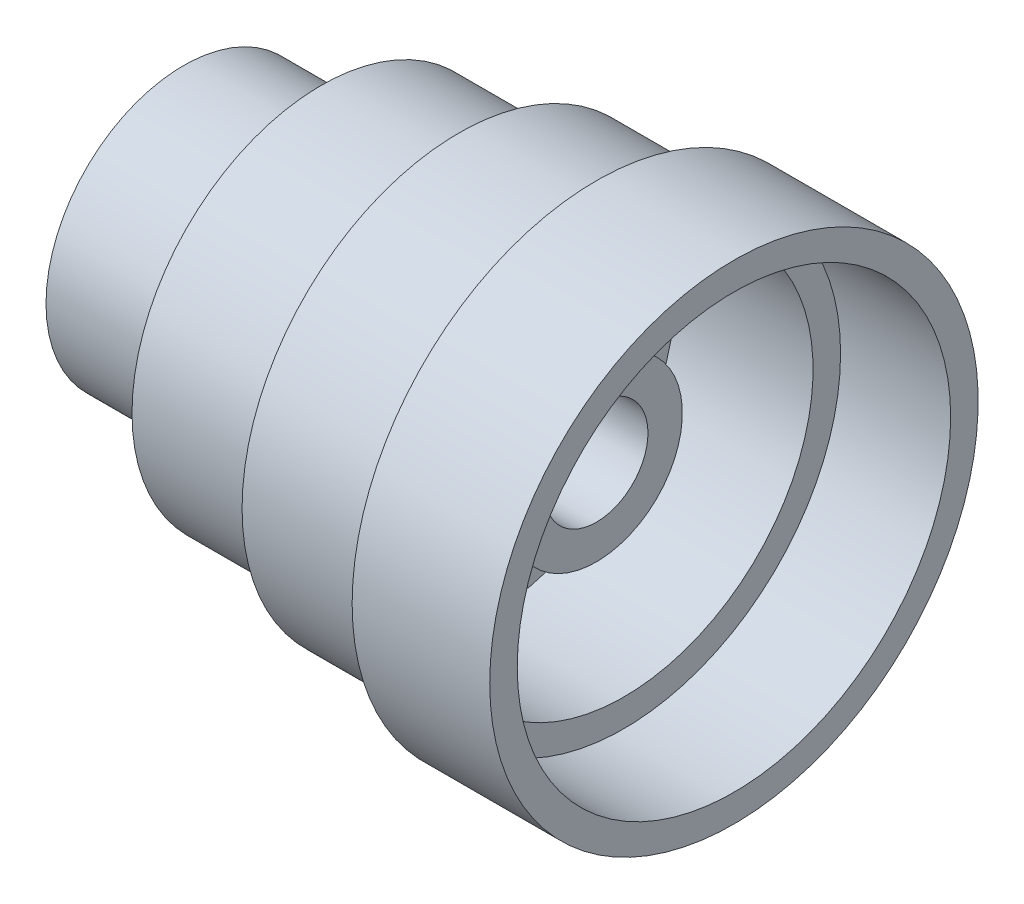
ISO-10303-21;
HEADER;
FILE_DESCRIPTION(('STEP AP214'),'2;1');
FILE_NAME('part.step','',(''),(''),'','','');
FILE_SCHEMA(('AUTOMOTIVE_DESIGN { 1 0 10303 214 1 1 1 1 }'));
ENDSEC;
DATA;
#1=APPLICATION_CONTEXT('core data for automotive mechanical design processes');
#2=APPLICATION_PROTOCOL_DEFINITION('international standard','automotive_design',2000,#1);
#3=PRODUCT_CONTEXT('',#1,'mechanical');
#4=PRODUCT('Part','Part','',(#3));
#5=PRODUCT_RELATED_PRODUCT_CATEGORY('part','',(#4));
#6=PRODUCT_DEFINITION_FORMATION('','',#4);
#7=PRODUCT_DEFINITION_CONTEXT('part definition',#1,'design');
#8=PRODUCT_DEFINITION('design','',#6,#7);
#9=PRODUCT_DEFINITION_SHAPE('','',#8);
#10=(LENGTH_UNIT() NAMED_UNIT(*) SI_UNIT(.MILLI.,.METRE.));
#11=(NAMED_UNIT(*) PLANE_ANGLE_UNIT() SI_UNIT($,.RADIAN.));
#12=(NAMED_UNIT(*) SI_UNIT($,.STERADIAN.) SOLID_ANGLE_UNIT());
#13=UNCERTAINTY_MEASURE_WITH_UNIT(LENGTH_MEASURE(1.E-05),#10,'distance_accuracy_value','');
#14=(GEOMETRIC_REPRESENTATION_CONTEXT(3) GLOBAL_UNCERTAINTY_ASSIGNED_CONTEXT((#13)) GLOBAL_UNIT_ASSIGNED_CONTEXT((#10,
#11,#12)) REPRESENTATION_CONTEXT('',''));
#15=CARTESIAN_POINT('',(0.,0.,0.));
#16=DIRECTION('',(0.,0.,1.));
#17=DIRECTION('',(1.,0.,0.));
#18=AXIS2_PLACEMENT_3D('',#15,#16,#17);
#19=CARTESIAN_POINT('',(-51.5789473684211,0.,0.));
#20=DIRECTION('',(-1.,0.,0.));
#21=DIRECTION('',(0.,0.,1.));
#22=AXIS2_PLACEMENT_3D('',#19,#20,#21);
#23=CYLINDRICAL_SURFACE('',#22,15.);
#24=CARTESIAN_POINT('',(0.,0.,0.));
#25=DIRECTION('',(-1.,0.,0.));
#26=DIRECTION('',(0.,0.,1.));
#27=AXIS2_PLACEMENT_3D('',#24,#25,#26);
#28=CIRCLE('',#27,15.);
#29=CARTESIAN_POINT('',(0.,14.6969384566991,-3.));
#30=VERTEX_POINT('',#29);
#31=CARTESIAN_POINT('',(0.,14.6969384566991,3.));
#32=VERTEX_POINT('',#31);
#33=EDGE_CURVE('E98',#30,#32,#28,.T.);
#34=ORIENTED_EDGE('',*,*,#33,.T.);
#35=DIRECTION('',(-1.,0.,0.));
#36=VECTOR('',#35,1.);
#37=CARTESIAN_POINT('',(-51.5789473684211,14.6969384566991,3.));
#38=LINE('',#37,#36);
#39=CARTESIAN_POINT('',(120.,14.6969384566991,3.));
#40=VERTEX_POINT('',#39);
#41=EDGE_CURVE('E110',#32,#40,#38,.F.);
#42=ORIENTED_EDGE('',*,*,#41,.T.);
#43=CARTESIAN_POINT('',(120.,0.,0.));
#44=DIRECTION('',(-1.,0.,0.));
#45=DIRECTION('',(0.,0.,1.));
#46=AXIS2_PLACEMENT_3D('',#43,#44,#45);
#47=CIRCLE('',#46,15.);
#48=CARTESIAN_POINT('',(120.,14.6969384566991,-3.));
#49=VERTEX_POINT('',#48);
#50=EDGE_CURVE('E46',#49,#40,#47,.T.);
#51=ORIENTED_EDGE('',*,*,#50,.F.);
#52=DIRECTION('',(-1.,0.,0.));
#53=VECTOR('',#52,1.);
#54=CARTESIAN_POINT('',(-51.5789473684211,14.6969384566991,-3.));
#55=LINE('',#54,#53);
#56=EDGE_CURVE('E102',#49,#30,#55,.T.);
#57=ORIENTED_EDGE('',*,*,#56,.T.);
#58=EDGE_LOOP('',(#34,#42,#51,#57));
#59=FACE_BOUND('',#58,.T.);
#60=ADVANCED_FACE('F39',(#59),#23,.F.);
#61=CARTESIAN_POINT('',(120.,25.,0.));
#62=DIRECTION('',(-1.,0.,0.));
#63=DIRECTION('',(0.,0.,1.));
#64=AXIS2_PLACEMENT_3D('',#61,#62,#63);
#65=PLANE('',#64);
#66=ORIENTED_EDGE('',*,*,#50,.T.);
#67=DIRECTION('',(0.,1.,0.));
#68=VECTOR('',#67,1.);
#69=CARTESIAN_POINT('',(120.,25.,3.));
#70=LINE('',#69,#68);
#71=CARTESIAN_POINT('',(120.,18.,3.));
#72=VERTEX_POINT('',#71);
#73=EDGE_CURVE('E58',#40,#72,#70,.T.);
#74=ORIENTED_EDGE('',*,*,#73,.T.);
#75=DIRECTION('',(0.,0.,-1.));
#76=VECTOR('',#75,1.);
#77=CARTESIAN_POINT('',(120.,18.,0.));
#78=LINE('',#77,#76);
#79=CARTESIAN_POINT('',(120.,18.,-3.));
#80=VERTEX_POINT('',#79);
#81=EDGE_CURVE('E87',#72,#80,#78,.T.);
#82=ORIENTED_EDGE('',*,*,#81,.T.);
#83=DIRECTION('',(0.,-1.,0.));
#84=VECTOR('',#83,1.);
#85=CARTESIAN_POINT('',(120.,25.,-3.));
#86=LINE('',#85,#84);
#87=EDGE_CURVE('E83',#80,#49,#86,.T.);
#88=ORIENTED_EDGE('',*,*,#87,.T.);
#89=EDGE_LOOP('',(#66,#74,#82,#88));
#90=FACE_BOUND('',#89,.T.);
#91=CARTESIAN_POINT('',(120.,0.,0.));
#92=DIRECTION('',(-1.,0.,0.));
#93=DIRECTION('',(0.,0.,1.));
#94=AXIS2_PLACEMENT_3D('',#91,#92,#93);
#95=CIRCLE('',#94,25.);
#96=CARTESIAN_POINT('',(120.,0.,25.));
#97=VERTEX_POINT('',#96);
#98=EDGE_CURVE('E154',#97,#97,#95,.T.);
#99=ORIENTED_EDGE('',*,*,#98,.F.);
#100=EDGE_LOOP('',(#99));
#101=FACE_BOUND('',#100,.T.);
#102=ADVANCED_FACE('F159',(#90,#101),#65,.F.);
#103=CARTESIAN_POINT('',(-51.5789473684211,0.,0.));
#104=DIRECTION('',(-1.,0.,0.));
#105=DIRECTION('',(0.,0.,1.));
#106=AXIS2_PLACEMENT_3D('',#103,#104,#105);
#107=CYLINDRICAL_SURFACE('',#106,25.);
#108=CARTESIAN_POINT('',(48.,0.,0.));
#109=DIRECTION('',(-1.,0.,0.));
#110=DIRECTION('',(0.,0.,1.));
#111=AXIS2_PLACEMENT_3D('',#108,#109,#110);
#112=CIRCLE('',#111,25.);
#113=CARTESIAN_POINT('',(48.,0.,25.));
#114=VERTEX_POINT('',#113);
#115=EDGE_CURVE('E155',#114,#114,#112,.T.);
#116=ORIENTED_EDGE('',*,*,#115,.F.);
#117=EDGE_LOOP('',(#116));
#118=FACE_BOUND('',#117,.T.);
#119=ORIENTED_EDGE('',*,*,#98,.T.);
#120=EDGE_LOOP('',(#119));
#121=FACE_BOUND('',#120,.T.);
#122=ADVANCED_FACE('F176',(#118,#121),#107,.T.);
#123=CARTESIAN_POINT('',(48.,40.,0.));
#124=DIRECTION('',(-1.,0.,0.));
#125=DIRECTION('',(0.,0.,1.));
#126=AXIS2_PLACEMENT_3D('',#123,#124,#125);
#127=PLANE('',#126);
#128=CARTESIAN_POINT('',(48.,0.,0.));
#129=DIRECTION('',(-1.,0.,0.));
#130=DIRECTION('',(0.,0.,1.));
#131=AXIS2_PLACEMENT_3D('',#128,#129,#130);
#132=CIRCLE('',#131,40.);
#133=CARTESIAN_POINT('',(48.,0.,40.));
#134=VERTEX_POINT('',#133);
#135=EDGE_CURVE('E149',#134,#134,#132,.T.);
#136=ORIENTED_EDGE('',*,*,#135,.F.);
#137=EDGE_LOOP('',(#136));
#138=FACE_BOUND('',#137,.T.);
#139=ORIENTED_EDGE('',*,*,#115,.T.);
#140=EDGE_LOOP('',(#139));
#141=FACE_BOUND('',#140,.T.);
#142=ADVANCED_FACE('F181',(#138,#141),#127,.F.);
#143=CARTESIAN_POINT('',(-51.5789473684211,0.,0.));
#144=DIRECTION('',(-1.,0.,0.));
#145=DIRECTION('',(0.,0.,1.));
#146=AXIS2_PLACEMENT_3D('',#143,#144,#145);
#147=CYLINDRICAL_SURFACE('',#146,40.);
#148=CARTESIAN_POINT('',(88.,0.,0.));
#149=DIRECTION('',(-1.,0.,0.));
#150=DIRECTION('',(0.,0.,1.));
#151=AXIS2_PLACEMENT_3D('',#148,#149,#150);
#152=CIRCLE('',#151,40.);
#153=CARTESIAN_POINT('',(88.,0.,40.));
#154=VERTEX_POINT('',#153);
#155=EDGE_CURVE('E148',#154,#154,#152,.T.);
#156=ORIENTED_EDGE('',*,*,#155,.F.);
#157=EDGE_LOOP('',(#156));
#158=FACE_BOUND('',#157,.T.);
#159=ORIENTED_EDGE('',*,*,#135,.T.);
#160=EDGE_LOOP('',(#159));
#161=FACE_BOUND('',#160,.T.);
#162=ADVANCED_FACE('F186',(#158,#161),#147,.F.);
#163=CARTESIAN_POINT('',(88.,55.,0.));
#164=DIRECTION('',(-1.,0.,0.));
#165=DIRECTION('',(0.,0.,1.));
#166=AXIS2_PLACEMENT_3D('',#163,#164,#165);
#167=PLANE('',#166);
#168=CARTESIAN_POINT('',(88.,0.,0.));
#169=DIRECTION('',(-1.,0.,0.));
#170=DIRECTION('',(0.,0.,1.));
#171=AXIS2_PLACEMENT_3D('',#168,#169,#170);
#172=CIRCLE('',#171,55.);
#173=CARTESIAN_POINT('',(88.,0.,55.));
#174=VERTEX_POINT('',#173);
#175=EDGE_CURVE('E141',#174,#174,#172,.T.);
#176=ORIENTED_EDGE('',*,*,#175,.F.);
#177=EDGE_LOOP('',(#176));
#178=FACE_BOUND('',#177,.T.);
#179=ORIENTED_EDGE('',*,*,#155,.T.);
#180=EDGE_LOOP('',(#179));
#181=FACE_BOUND('',#180,.T.);
#182=ADVANCED_FACE('F195',(#178,#181),#167,.F.);
#183=CARTESIAN_POINT('',(-51.5789473684211,0.,0.));
#184=DIRECTION('',(-1.,0.,0.));
#185=DIRECTION('',(0.,0.,1.));
#186=AXIS2_PLACEMENT_3D('',#183,#184,#185);
#187=CYLINDRICAL_SURFACE('',#186,55.);
#188=CARTESIAN_POINT('',(128.,0.,0.));
#189=DIRECTION('',(-1.,0.,0.));
#190=DIRECTION('',(0.,0.,1.));
#191=AXIS2_PLACEMENT_3D('',#188,#189,#190);
#192=CIRCLE('',#191,55.);
#193=CARTESIAN_POINT('',(128.,0.,55.));
#194=VERTEX_POINT('',#193);
#195=EDGE_CURVE('E138',#194,#194,#192,.T.);
#196=ORIENTED_EDGE('',*,*,#195,.F.);
#197=EDGE_LOOP('',(#196));
#198=FACE_BOUND('',#197,.T.);
#199=ORIENTED_EDGE('',*,*,#175,.T.);
#200=EDGE_LOOP('',(#199));
#201=FACE_BOUND('',#200,.T.);
#202=ADVANCED_FACE('F197',(#198,#201),#187,.F.);
#203=CARTESIAN_POINT('',(128.,63.,0.));
#204=DIRECTION('',(-1.,0.,0.));
#205=DIRECTION('',(0.,0.,1.));
#206=AXIS2_PLACEMENT_3D('',#203,#204,#205);
#207=PLANE('',#206);
#208=CARTESIAN_POINT('',(128.,0.,0.));
#209=DIRECTION('',(-1.,0.,0.));
#210=DIRECTION('',(0.,0.,1.));
#211=AXIS2_PLACEMENT_3D('',#208,#209,#210);
#212=CIRCLE('',#211,63.);
#213=CARTESIAN_POINT('',(128.,0.,63.));
#214=VERTEX_POINT('',#213);
#215=EDGE_CURVE('E139',#214,#214,#212,.T.);
#216=ORIENTED_EDGE('',*,*,#215,.F.);
#217=EDGE_LOOP('',(#216));
#218=FACE_BOUND('',#217,.T.);
#219=ORIENTED_EDGE('',*,*,#195,.T.);
#220=EDGE_LOOP('',(#219));
#221=FACE_BOUND('',#220,.T.);
#222=ADVANCED_FACE('F203',(#218,#221),#207,.F.);
#223=CARTESIAN_POINT('',(-51.5789473684211,0.,0.));
#224=DIRECTION('',(-1.,0.,0.));
#225=DIRECTION('',(0.,0.,1.));
#226=AXIS2_PLACEMENT_3D('',#223,#224,#225);
#227=CYLINDRICAL_SURFACE('',#226,63.);
#228=CARTESIAN_POINT('',(160.,0.,0.));
#229=DIRECTION('',(-1.,0.,0.));
#230=DIRECTION('',(0.,0.,1.));
#231=AXIS2_PLACEMENT_3D('',#228,#229,#230);
#232=CIRCLE('',#231,63.);
#233=CARTESIAN_POINT('',(160.,0.,63.));
#234=VERTEX_POINT('',#233);
#235=EDGE_CURVE('E131',#234,#234,#232,.T.);
#236=ORIENTED_EDGE('',*,*,#235,.F.);
#237=EDGE_LOOP('',(#236));
#238=FACE_BOUND('',#237,.T.);
#239=ORIENTED_EDGE('',*,*,#215,.T.);
#240=EDGE_LOOP('',(#239));
#241=FACE_BOUND('',#240,.T.);
#242=ADVANCED_FACE('F202',(#238,#241),#227,.F.);
#243=CARTESIAN_POINT('',(160.,71.,0.));
#244=DIRECTION('',(-1.,0.,0.));
#245=DIRECTION('',(0.,0.,1.));
#246=AXIS2_PLACEMENT_3D('',#243,#244,#245);
#247=PLANE('',#246);
#248=CARTESIAN_POINT('',(160.,0.,0.));
#249=DIRECTION('',(-1.,0.,0.));
#250=DIRECTION('',(0.,0.,1.));
#251=AXIS2_PLACEMENT_3D('',#248,#249,#250);
#252=CIRCLE('',#251,71.);
#253=CARTESIAN_POINT('',(160.,0.,71.));
#254=VERTEX_POINT('',#253);
#255=EDGE_CURVE('E132',#254,#254,#252,.T.);
#256=ORIENTED_EDGE('',*,*,#255,.F.);
#257=EDGE_LOOP('',(#256));
#258=FACE_BOUND('',#257,.T.);
#259=ORIENTED_EDGE('',*,*,#235,.T.);
#260=EDGE_LOOP('',(#259));
#261=FACE_BOUND('',#260,.T.);
#262=ADVANCED_FACE('F207',(#258,#261),#247,.F.);
#263=CARTESIAN_POINT('',(-51.5789473684211,0.,0.));
#264=DIRECTION('',(-1.,0.,0.));
#265=DIRECTION('',(0.,0.,1.));
#266=AXIS2_PLACEMENT_3D('',#263,#264,#265);
#267=CYLINDRICAL_SURFACE('',#266,71.);
#268=CARTESIAN_POINT('',(120.,0.,0.));
#269=DIRECTION('',(-1.,0.,0.));
#270=DIRECTION('',(0.,0.,1.));
#271=AXIS2_PLACEMENT_3D('',#268,#269,#270);
#272=CIRCLE('',#271,71.);
#273=CARTESIAN_POINT('',(120.,0.,71.));
#274=VERTEX_POINT('',#273);
#275=EDGE_CURVE('E126',#274,#274,#272,.T.);
#276=ORIENTED_EDGE('',*,*,#275,.F.);
#277=EDGE_LOOP('',(#276));
#278=FACE_BOUND('',#277,.T.);
#279=ORIENTED_EDGE('',*,*,#255,.T.);
#280=EDGE_LOOP('',(#279));
#281=FACE_BOUND('',#280,.T.);
#282=ADVANCED_FACE('F213',(#278,#281),#267,.T.);
#283=CARTESIAN_POINT('',(120.,63.,0.));
#284=DIRECTION('',(1.,0.,0.));
#285=DIRECTION('',(0.,0.,-1.));
#286=AXIS2_PLACEMENT_3D('',#283,#284,#285);
#287=PLANE('',#286);
#288=CARTESIAN_POINT('',(120.,0.,0.));
#289=DIRECTION('',(-1.,0.,0.));
#290=DIRECTION('',(0.,0.,1.));
#291=AXIS2_PLACEMENT_3D('',#288,#289,#290);
#292=CIRCLE('',#291,63.);
#293=CARTESIAN_POINT('',(120.,0.,63.));
#294=VERTEX_POINT('',#293);
#295=EDGE_CURVE('E123',#294,#294,#292,.T.);
#296=ORIENTED_EDGE('',*,*,#295,.F.);
#297=EDGE_LOOP('',(#296));
#298=FACE_BOUND('',#297,.T.);
#299=ORIENTED_EDGE('',*,*,#275,.T.);
#300=EDGE_LOOP('',(#299));
#301=FACE_BOUND('',#300,.T.);
#302=ADVANCED_FACE('F220',(#298,#301),#287,.F.);
#303=CARTESIAN_POINT('',(-51.5789473684211,0.,0.));
#304=DIRECTION('',(-1.,0.,0.));
#305=DIRECTION('',(0.,0.,1.));
#306=AXIS2_PLACEMENT_3D('',#303,#304,#305);
#307=CYLINDRICAL_SURFACE('',#306,63.);
#308=CARTESIAN_POINT('',(80.,0.,0.));
#309=DIRECTION('',(-1.,0.,0.));
#310=DIRECTION('',(0.,0.,1.));
#311=AXIS2_PLACEMENT_3D('',#308,#309,#310);
#312=CIRCLE('',#311,63.);
#313=CARTESIAN_POINT('',(80.,0.,63.));
#314=VERTEX_POINT('',#313);
#315=EDGE_CURVE('E124',#314,#314,#312,.T.);
#316=ORIENTED_EDGE('',*,*,#315,.F.);
#317=EDGE_LOOP('',(#316));
#318=FACE_BOUND('',#317,.T.);
#319=ORIENTED_EDGE('',*,*,#295,.T.);
#320=EDGE_LOOP('',(#319));
#321=FACE_BOUND('',#320,.T.);
#322=ADVANCED_FACE('F222',(#318,#321),#307,.T.);
#323=CARTESIAN_POINT('',(80.,55.,0.));
#324=DIRECTION('',(1.,0.,0.));
#325=DIRECTION('',(0.,0.,-1.));
#326=AXIS2_PLACEMENT_3D('',#323,#324,#325);
#327=PLANE('',#326);
#328=CARTESIAN_POINT('',(80.,0.,0.));
#329=DIRECTION('',(-1.,0.,0.));
#330=DIRECTION('',(0.,0.,1.));
#331=AXIS2_PLACEMENT_3D('',#328,#329,#330);
#332=CIRCLE('',#331,55.);
#333=CARTESIAN_POINT('',(80.,0.,55.));
#334=VERTEX_POINT('',#333);
#335=EDGE_CURVE('E116',#334,#334,#332,.T.);
#336=ORIENTED_EDGE('',*,*,#335,.F.);
#337=EDGE_LOOP('',(#336));
#338=FACE_BOUND('',#337,.T.);
#339=ORIENTED_EDGE('',*,*,#315,.T.);
#340=EDGE_LOOP('',(#339));
#341=FACE_BOUND('',#340,.T.);
#342=ADVANCED_FACE('F223',(#338,#341),#327,.F.);
#343=CARTESIAN_POINT('',(-51.5789473684211,0.,0.));
#344=DIRECTION('',(-1.,0.,0.));
#345=DIRECTION('',(0.,0.,1.));
#346=AXIS2_PLACEMENT_3D('',#343,#344,#345);
#347=CYLINDRICAL_SURFACE('',#346,55.);
#348=CARTESIAN_POINT('',(40.,0.,0.));
#349=DIRECTION('',(-1.,0.,0.));
#350=DIRECTION('',(0.,0.,1.));
#351=AXIS2_PLACEMENT_3D('',#348,#349,#350);
#352=CIRCLE('',#351,55.);
#353=CARTESIAN_POINT('',(40.,0.,55.));
#354=VERTEX_POINT('',#353);
#355=EDGE_CURVE('E117',#354,#354,#352,.T.);
#356=ORIENTED_EDGE('',*,*,#355,.F.);
#357=EDGE_LOOP('',(#356));
#358=FACE_BOUND('',#357,.T.);
#359=ORIENTED_EDGE('',*,*,#335,.T.);
#360=EDGE_LOOP('',(#359));
#361=FACE_BOUND('',#360,.T.);
#362=ADVANCED_FACE('F226',(#358,#361),#347,.T.);
#363=CARTESIAN_POINT('',(40.,40.,0.));
#364=DIRECTION('',(1.,0.,0.));
#365=DIRECTION('',(0.,0.,-1.));
#366=AXIS2_PLACEMENT_3D('',#363,#364,#365);
#367=PLANE('',#366);
#368=CARTESIAN_POINT('',(40.,0.,0.));
#369=DIRECTION('',(-1.,0.,0.));
#370=DIRECTION('',(0.,0.,1.));
#371=AXIS2_PLACEMENT_3D('',#368,#369,#370);
#372=CIRCLE('',#371,40.);
#373=CARTESIAN_POINT('',(40.,0.,40.));
#374=VERTEX_POINT('',#373);
#375=EDGE_CURVE('E114',#374,#374,#372,.T.);
#376=ORIENTED_EDGE('',*,*,#375,.F.);
#377=EDGE_LOOP('',(#376));
#378=FACE_BOUND('',#377,.T.);
#379=ORIENTED_EDGE('',*,*,#355,.T.);
#380=EDGE_LOOP('',(#379));
#381=FACE_BOUND('',#380,.T.);
#382=ADVANCED_FACE('F235',(#378,#381),#367,.F.);
#383=CARTESIAN_POINT('',(-51.5789473684211,0.,0.));
#384=DIRECTION('',(-1.,0.,0.));
#385=DIRECTION('',(0.,0.,1.));
#386=AXIS2_PLACEMENT_3D('',#383,#384,#385);
#387=CYLINDRICAL_SURFACE('',#386,40.);
#388=CARTESIAN_POINT('',(0.,0.,0.));
#389=DIRECTION('',(-1.,0.,0.));
#390=DIRECTION('',(0.,0.,1.));
#391=AXIS2_PLACEMENT_3D('',#388,#389,#390);
#392=CIRCLE('',#391,40.);
#393=CARTESIAN_POINT('',(0.,0.,40.));
#394=VERTEX_POINT('',#393);
#395=EDGE_CURVE('E109',#394,#394,#392,.T.);
#396=ORIENTED_EDGE('',*,*,#395,.F.);
#397=EDGE_LOOP('',(#396));
#398=FACE_BOUND('',#397,.T.);
#399=ORIENTED_EDGE('',*,*,#375,.T.);
#400=EDGE_LOOP('',(#399));
#401=FACE_BOUND('',#400,.T.);
#402=ADVANCED_FACE('F172',(#398,#401),#387,.T.);
#403=CARTESIAN_POINT('',(0.,40.,0.));
#404=DIRECTION('',(1.,0.,0.));
#405=DIRECTION('',(0.,0.,-1.));
#406=AXIS2_PLACEMENT_3D('',#403,#404,#405);
#407=PLANE('',#406);
#408=DIRECTION('',(0.,0.,-1.));
#409=VECTOR('',#408,1.);
#410=CARTESIAN_POINT('',(0.,18.,-3.));
#411=LINE('',#410,#409);
#412=CARTESIAN_POINT('',(0.,18.,3.));
#413=VERTEX_POINT('',#412);
#414=CARTESIAN_POINT('',(0.,18.,-3.));
#415=VERTEX_POINT('',#414);
#416=EDGE_CURVE('E89',#413,#415,#411,.T.);
#417=ORIENTED_EDGE('',*,*,#416,.F.);
#418=DIRECTION('',(0.,-1.,0.));
#419=VECTOR('',#418,1.);
#420=CARTESIAN_POINT('',(0.,40.,3.));
#421=LINE('',#420,#419);
#422=EDGE_CURVE('E11',#413,#32,#421,.T.);
#423=ORIENTED_EDGE('',*,*,#422,.T.);
#424=ORIENTED_EDGE('',*,*,#33,.F.);
#425=DIRECTION('',(0.,-1.,0.));
#426=VECTOR('',#425,1.);
#427=CARTESIAN_POINT('',(0.,18.,-3.));
#428=LINE('',#427,#426);
#429=EDGE_CURVE('E84',#415,#30,#428,.T.);
#430=ORIENTED_EDGE('',*,*,#429,.F.);
#431=EDGE_LOOP('',(#417,#423,#424,#430));
#432=FACE_BOUND('',#431,.T.);
#433=ORIENTED_EDGE('',*,*,#395,.T.);
#434=EDGE_LOOP('',(#433));
#435=FACE_BOUND('',#434,.T.);
#436=ADVANCED_FACE('F92',(#432,#435),#407,.F.);
#437=CARTESIAN_POINT('',(211.,18.,3.));
#438=DIRECTION('',(0.,0.,1.));
#439=DIRECTION('',(0.,-1.,0.));
#440=AXIS2_PLACEMENT_3D('',#437,#438,#439);
#441=PLANE('',#440);
#442=ORIENTED_EDGE('',*,*,#422,.F.);
#443=DIRECTION('',(-1.,0.,0.));
#444=VECTOR('',#443,1.);
#445=CARTESIAN_POINT('',(211.,18.,3.));
#446=LINE('',#445,#444);
#447=EDGE_CURVE('E52',#72,#413,#446,.T.);
#448=ORIENTED_EDGE('',*,*,#447,.F.);
#449=ORIENTED_EDGE('',*,*,#73,.F.);
#450=ORIENTED_EDGE('',*,*,#41,.F.);
#451=EDGE_LOOP('',(#442,#448,#449,#450));
#452=FACE_BOUND('',#451,.T.);
#453=ADVANCED_FACE('F162',(#452),#441,.F.);
#454=CARTESIAN_POINT('',(211.,18.,-3.));
#455=DIRECTION('',(0.,0.,-1.));
#456=DIRECTION('',(0.,1.,0.));
#457=AXIS2_PLACEMENT_3D('',#454,#455,#456);
#458=PLANE('',#457);
#459=ORIENTED_EDGE('',*,*,#87,.F.);
#460=DIRECTION('',(-1.,0.,0.));
#461=VECTOR('',#460,1.);
#462=CARTESIAN_POINT('',(211.,18.,-3.));
#463=LINE('',#462,#461);
#464=EDGE_CURVE('E76',#80,#415,#463,.T.);
#465=ORIENTED_EDGE('',*,*,#464,.T.);
#466=ORIENTED_EDGE('',*,*,#429,.T.);
#467=ORIENTED_EDGE('',*,*,#56,.F.);
#468=EDGE_LOOP('',(#459,#465,#466,#467));
#469=FACE_BOUND('',#468,.T.);
#470=ADVANCED_FACE('F78',(#469),#458,.F.);
#471=CARTESIAN_POINT('',(211.,18.,-3.));
#472=DIRECTION('',(0.,1.,0.));
#473=DIRECTION('',(0.,0.,1.));
#474=AXIS2_PLACEMENT_3D('',#471,#472,#473);
#475=PLANE('',#474);
#476=ORIENTED_EDGE('',*,*,#447,.T.);
#477=ORIENTED_EDGE('',*,*,#416,.T.);
#478=ORIENTED_EDGE('',*,*,#464,.F.);
#479=ORIENTED_EDGE('',*,*,#81,.F.);
#480=EDGE_LOOP('',(#476,#477,#478,#479));
#481=FACE_BOUND('',#480,.T.);
#482=ADVANCED_FACE('F93',(#481),#475,.F.);
#483=CLOSED_SHELL('',(#60,#102,#122,#142,#162,#182,#202,#222,#242,#262,#282,#302,#322,#342,#362,
#382,#402,#436,#453,#470,#482));
#484=MANIFOLD_SOLID_BREP('B2',#483);
#485=ADVANCED_BREP_SHAPE_REPRESENTATION('',(#18,#484),#14);
#486=SHAPE_DEFINITION_REPRESENTATION(#9,#485);
ENDSEC;
END-ISO-10303-21;
